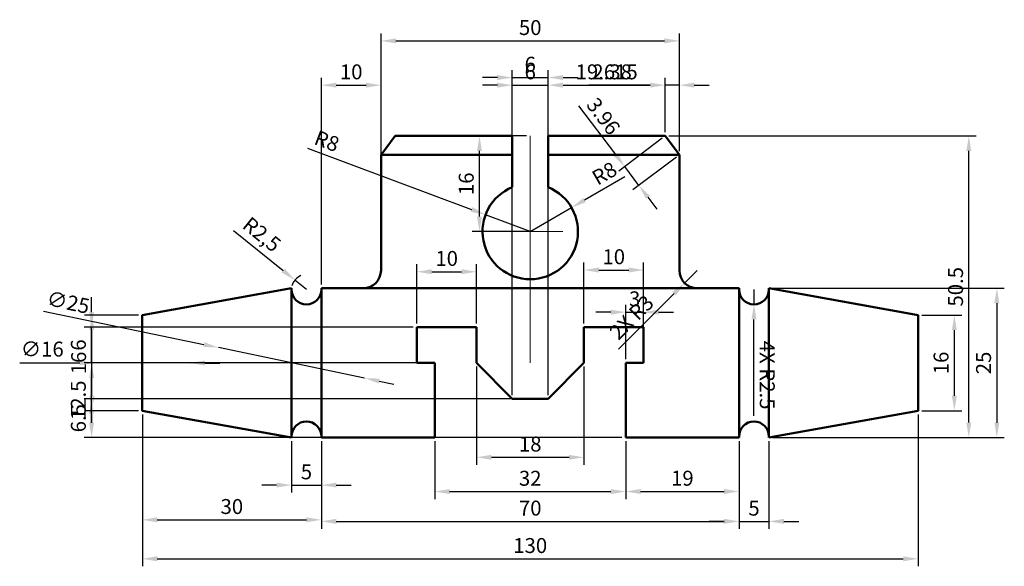
# Model space of a CAD drawing. Units: millimetres. Extents: x 4064 to 4229, y 716 to 807.
import ezdxf

# ---------------------------------------------------------------- set-up
doc = ezdxf.new("R2010")
doc.units = ezdxf.units.MM
doc.linetypes.add('CENTER', pattern=[50.8, 31.75, -6.35, 6.35, -6.35])
for name, color, linetype, lineweight in [('M-CNTR', 4, 'CENTER', 18), ('M-DIMS', 2, 'Continuous', 25), ('M-OUTL', 7, 'Continuous', 50)]:
    doc.layers.add(name, color=color, linetype=linetype, lineweight=lineweight)
doc.styles.get("Standard").update_dxf_attribs({"font": 'arial.ttf'})
doc.dimstyles.new('ISO-25', dxfattribs={"dimtxt": 2.5, "dimasz": 2.5, "dimexe": 1.25, "dimexo": 0.625, "dimtad": 1, "dimtxsty": 'Standard', "dimcen": 2.5, "dimadec": 0, "dimazin": 0, "dimtfac": 1, "dimtmove": 0, "dimatfit": 3, "dimfxl": 1, "dimarcsym": 0})

# ---------------------------------------------------------------- blocks, each defined once
blk = doc.blocks.new('*D1')
at = {"layer": 'Defpoints', "color": 0, "transparency": 16777216}
for p in [(4174.35, 803.87), (4124.35, 784.79), (4174.35, 784.79)]:
    blk.add_point(p, dxfattribs=at)
at = {"layer": 'M-DIMS', "color": 0, "lineweight": -2, "transparency": 16777216}
for p, q in [((4124.35, 785.42), (4124.35, 805.12)), ((4126.85, 803.87), (4171.85, 803.87)), ((4174.35, 785.42), (4174.35, 805.12))]:
    blk.add_line(p, q, dxfattribs=at)
at = {"layer": 'M-DIMS', "color": 0, "transparency": 16777216}
for points in [[(4126.85, 804.29), (4126.85, 803.45), (4124.35, 803.87)], [(4171.85, 804.29), (4171.85, 803.45), (4174.35, 803.87)]]:
    blk.add_solid(points, dxfattribs=at)
at = {"layer": 'M-DIMS', "color": 0, "transparency": 16777216, "insert": (4149.35, 805.77), "char_height": 2.5, "attachment_point": 5}
blk.add_mtext('50', dxfattribs=at)
blk = doc.blocks.new('*D2')
at = {"layer": 'Defpoints', "color": 0, "transparency": 16777216}
for p in [(4152.35, 797.73), (4146.35, 787.95), (4152.35, 787.95)]:
    blk.add_point(p, dxfattribs=at)
at = {"layer": 'M-DIMS', "color": 0, "lineweight": -2, "transparency": 16777216}
for p, q in [((4146.35, 788.58), (4146.35, 798.98)), ((4152.35, 788.58), (4152.35, 798.98)), ((4143.85, 797.73), (4141.35, 797.73)), ((4146.35, 797.73), (4152.35, 797.73)), ((4154.85, 797.73), (4157.35, 797.73))]:
    blk.add_line(p, q, dxfattribs=at)
at = {"layer": 'M-DIMS', "color": 0, "transparency": 16777216}
for points in [[(4143.85, 798.15), (4143.85, 797.32), (4146.35, 797.73)], [(4154.85, 798.15), (4154.85, 797.32), (4152.35, 797.73)]]:
    blk.add_solid(points, dxfattribs=at)
at = {"layer": 'M-DIMS', "color": 0, "transparency": 16777216, "insert": (4149.35, 799.63), "char_height": 2.5, "attachment_point": 5}
blk.add_mtext('6', dxfattribs=at)
blk = doc.blocks.new('*D3')
at = {"layer": 'Defpoints', "color": 0, "transparency": 16777216}
for p in [(4140.35, 749.95), (4158.35, 749.95), (4158.35, 734.15)]:
    blk.add_point(p, dxfattribs=at)
at = {"layer": 'M-DIMS', "color": 0, "lineweight": -2, "transparency": 16777216}
for p, q in [((4140.35, 749.33), (4140.35, 732.9)), ((4158.35, 749.33), (4158.35, 732.9)), ((4142.85, 734.15), (4155.85, 734.15))]:
    blk.add_line(p, q, dxfattribs=at)
at = {"layer": 'M-DIMS', "color": 0, "transparency": 16777216}
for points in [[(4142.85, 734.57), (4142.85, 733.74), (4140.35, 734.15)], [(4155.85, 734.57), (4155.85, 733.74), (4158.35, 734.15)]]:
    blk.add_solid(points, dxfattribs=at)
at = {"layer": 'M-DIMS', "color": 0, "transparency": 16777216, "insert": (4149.35, 736.05), "char_height": 2.5, "attachment_point": 5}
blk.add_mtext('18', dxfattribs=at)
blk = doc.blocks.new('*D4')
at = {"layer": 'Defpoints', "color": 0, "transparency": 16777216}
for p in [(4133.35, 737.45), (4165.35, 737.45), (4165.35, 728.42)]:
    blk.add_point(p, dxfattribs=at)
at = {"layer": 'M-DIMS', "color": 0, "lineweight": -2, "transparency": 16777216}
for p, q in [((4133.35, 736.83), (4133.35, 727.17)), ((4165.35, 736.83), (4165.35, 727.17)), ((4135.85, 728.42), (4162.85, 728.42))]:
    blk.add_line(p, q, dxfattribs=at)
at = {"layer": 'M-DIMS', "color": 0, "transparency": 16777216}
for points in [[(4135.85, 728.84), (4135.85, 728), (4133.35, 728.42)], [(4162.85, 728.84), (4162.85, 728), (4165.35, 728.42)]]:
    blk.add_solid(points, dxfattribs=at)
at = {"layer": 'M-DIMS', "color": 0, "transparency": 16777216, "insert": (4149.35, 730.32), "char_height": 2.5, "attachment_point": 5}
blk.add_mtext('32', dxfattribs=at)
blk = doc.blocks.new('*D5')
at = {"layer": 'Defpoints', "color": 0, "transparency": 16777216}
for p in [(4165.35, 737.45), (4184.35, 737.45), (4184.35, 728.43)]:
    blk.add_point(p, dxfattribs=at)
at = {"layer": 'M-DIMS', "color": 0, "lineweight": -2, "transparency": 16777216}
for p, q in [((4165.35, 736.83), (4165.35, 727.18)), ((4184.35, 736.83), (4184.35, 727.18)), ((4167.85, 728.43), (4181.85, 728.43))]:
    blk.add_line(p, q, dxfattribs=at)
at = {"layer": 'M-DIMS', "color": 0, "transparency": 16777216}
for points in [[(4167.85, 728.85), (4167.85, 728.01), (4165.35, 728.43)], [(4181.85, 728.85), (4181.85, 728.01), (4184.35, 728.43)]]:
    blk.add_solid(points, dxfattribs=at)
at = {"layer": 'M-DIMS', "color": 0, "transparency": 16777216, "insert": (4174.85, 730.33), "char_height": 2.5, "attachment_point": 5}
blk.add_mtext('19', dxfattribs=at)
blk = doc.blocks.new('*D6')
at = {"layer": 'Defpoints', "color": 0, "transparency": 16777216}
for p in [(4114.35, 737.45), (4184.35, 737.45), (4184.35, 723.43)]:
    blk.add_point(p, dxfattribs=at)
at = {"layer": 'M-DIMS', "color": 0, "lineweight": -2, "transparency": 16777216}
for p, q in [((4114.35, 736.83), (4114.35, 722.18)), ((4184.35, 736.83), (4184.35, 722.18)), ((4116.85, 723.43), (4181.85, 723.43))]:
    blk.add_line(p, q, dxfattribs=at)
at = {"layer": 'M-DIMS', "color": 0, "transparency": 16777216}
for points in [[(4116.85, 723.85), (4116.85, 723.01), (4114.35, 723.43)], [(4181.85, 723.85), (4181.85, 723.01), (4184.35, 723.43)]]:
    blk.add_solid(points, dxfattribs=at)
at = {"layer": 'M-DIMS', "color": 0, "transparency": 16777216, "insert": (4149.35, 725.33), "char_height": 2.5, "attachment_point": 5}
blk.add_mtext('70', dxfattribs=at)
blk = doc.blocks.new('*D7')
at = {"layer": 'Defpoints', "color": 0, "transparency": 16777216}
for p in [(4184.35, 737.45), (4189.35, 737.45), (4189.35, 723.42)]:
    blk.add_point(p, dxfattribs=at)
at = {"layer": 'M-DIMS', "color": 0, "lineweight": -2, "transparency": 16777216}
for p, q in [((4184.35, 736.83), (4184.35, 722.17)), ((4189.35, 736.83), (4189.35, 722.17)), ((4181.85, 723.42), (4179.35, 723.42)), ((4184.35, 723.42), (4189.35, 723.42)), ((4191.85, 723.42), (4194.35, 723.42))]:
    blk.add_line(p, q, dxfattribs=at)
at = {"layer": 'M-DIMS', "color": 0, "transparency": 16777216}
for points in [[(4181.85, 723.84), (4181.85, 723.01), (4184.35, 723.42)], [(4191.85, 723.84), (4191.85, 723.01), (4189.35, 723.42)]]:
    blk.add_solid(points, dxfattribs=at)
at = {"layer": 'M-DIMS', "color": 0, "transparency": 16777216, "insert": (4186.85, 725.32), "char_height": 2.5, "attachment_point": 5}
blk.add_mtext('5', dxfattribs=at)
blk = doc.blocks.new('*D8')
at = {"layer": 'Defpoints', "color": 0, "transparency": 16777216}
for p in [(4109.35, 737.46), (4114.35, 737.45), (4114.35, 729.5)]:
    blk.add_point(p, dxfattribs=at)
at = {"layer": 'M-DIMS', "color": 0, "lineweight": -2, "transparency": 16777216}
for p, q in [((4109.35, 736.83), (4109.35, 728.25)), ((4114.35, 736.83), (4114.35, 728.25)), ((4106.85, 729.5), (4104.35, 729.5)), ((4109.35, 729.5), (4114.35, 729.5)), ((4116.85, 729.5), (4119.35, 729.5))]:
    blk.add_line(p, q, dxfattribs=at)
at = {"layer": 'M-DIMS', "color": 0, "transparency": 16777216}
for points in [[(4106.85, 729.92), (4106.85, 729.09), (4109.35, 729.5)], [(4116.85, 729.92), (4116.85, 729.09), (4114.35, 729.5)]]:
    blk.add_solid(points, dxfattribs=at)
at = {"layer": 'M-DIMS', "color": 0, "transparency": 16777216, "insert": (4111.85, 731.4), "char_height": 2.5, "attachment_point": 5}
blk.add_mtext('5', dxfattribs=at)
blk = doc.blocks.new('*D9')
at = {"layer": 'Defpoints', "color": 0, "transparency": 16777216}
for p in [(4084.35, 741.95), (4114.35, 737.45), (4114.35, 723.69)]:
    blk.add_point(p, dxfattribs=at)
at = {"layer": 'M-DIMS', "color": 0, "lineweight": -2, "transparency": 16777216}
for p, q in [((4084.35, 741.33), (4084.35, 722.44)), ((4114.35, 736.83), (4114.35, 722.44)), ((4086.85, 723.69), (4111.85, 723.69))]:
    blk.add_line(p, q, dxfattribs=at)
at = {"layer": 'M-DIMS', "color": 0, "transparency": 16777216}
for points in [[(4086.85, 724.1), (4086.85, 723.27), (4084.35, 723.69)], [(4111.85, 724.1), (4111.85, 723.27), (4114.35, 723.69)]]:
    blk.add_solid(points, dxfattribs=at)
at = {"layer": 'M-DIMS', "color": 0, "transparency": 16777216, "insert": (4099.35, 725.59), "char_height": 2.5, "attachment_point": 5}
blk.add_mtext('30', dxfattribs=at)
blk = doc.blocks.new('*D10')
at = {"layer": 'Defpoints', "color": 0, "transparency": 16777216}
for p in [(4084.35, 741.95), (4214.35, 741.95), (4214.35, 717.16)]:
    blk.add_point(p, dxfattribs=at)
at = {"layer": 'M-DIMS', "color": 0, "lineweight": -2, "transparency": 16777216}
for p, q in [((4084.35, 741.33), (4084.35, 715.91)), ((4214.35, 741.33), (4214.35, 715.91)), ((4086.85, 717.16), (4211.85, 717.16))]:
    blk.add_line(p, q, dxfattribs=at)
at = {"layer": 'M-DIMS', "color": 0, "transparency": 16777216}
for points in [[(4086.85, 717.58), (4086.85, 716.74), (4084.35, 717.16)], [(4211.85, 717.58), (4211.85, 716.74), (4214.35, 717.16)]]:
    blk.add_solid(points, dxfattribs=at)
at = {"layer": 'M-DIMS', "color": 0, "transparency": 16777216, "insert": (4149.35, 719.06), "char_height": 2.5, "attachment_point": 5}
blk.add_mtext('130', dxfattribs=at)
blk = doc.blocks.new('*D11')
at = {"layer": 'Defpoints', "color": 0, "transparency": 16777216}
for p in [(4076.35, 749.97), (4092.35, 749.94)]:
    blk.add_point(p, dxfattribs=at)
at = {"layer": 'M-DIMS', "color": 0, "lineweight": -2, "transparency": 16777216}
for p, q in [((4063.8, 749.99), (4073.85, 749.97)), ((4092.35, 749.94), (4076.35, 749.97)), ((4094.85, 749.94), (4097.35, 749.93))]:
    blk.add_line(p, q, dxfattribs=at)
at = {"layer": 'M-DIMS', "color": 0, "transparency": 16777216}
for points in [[(4073.85, 750.39), (4073.85, 749.55), (4076.35, 749.97)], [(4094.85, 750.35), (4094.85, 749.52), (4092.35, 749.94)]]:
    blk.add_solid(points, dxfattribs=at)
at = {"layer": 'M-DIMS', "color": 0, "transparency": 16777216, "insert": (4067.58, 751.95), "char_height": 2.5, "attachment_point": 5, "rotation": 359.9089}
blk.add_mtext('∅16', dxfattribs=at)
blk = doc.blocks.new('*D12')
at = {"layer": 'Defpoints', "color": 0, "transparency": 16777216}
for p in [(4097.11, 752.52), (4121.58, 747.42)]:
    blk.add_point(p, dxfattribs=at)
at = {"layer": 'M-DIMS', "color": 0, "lineweight": -2, "transparency": 16777216}
for p, q in [((4067.77, 758.64), (4094.66, 753.03)), ((4121.58, 747.42), (4097.11, 752.52)), ((4124.03, 746.91), (4126.48, 746.4))]:
    blk.add_line(p, q, dxfattribs=at)
at = {"layer": 'M-DIMS', "color": 0, "transparency": 16777216}
for points in [[(4094.75, 753.44), (4094.58, 752.63), (4097.11, 752.52)], [(4124.12, 747.32), (4123.95, 746.51), (4121.58, 747.42)]]:
    blk.add_solid(points, dxfattribs=at)
at = {"layer": 'M-DIMS', "color": 0, "transparency": 16777216, "insert": (4071.87, 759.79), "char_height": 2.5, "attachment_point": 5, "rotation": 348.232}
blk.add_mtext('∅25', dxfattribs=at)
blk = doc.blocks.new('*D13')
at = {"layer": 'Defpoints', "color": 0, "transparency": 16777216}
for p in [(4075.9, 757.95), (4084.35, 757.95), (4084.35, 741.95)]:
    blk.add_point(p, dxfattribs=at)
at = {"layer": 'M-DIMS', "color": 0, "lineweight": -2, "transparency": 16777216}
for p, q in [((4083.72, 757.95), (4074.65, 757.95)), ((4075.9, 744.45), (4075.9, 755.45)), ((4083.72, 741.95), (4074.65, 741.95))]:
    blk.add_line(p, q, dxfattribs=at)
at = {"layer": 'M-DIMS', "color": 0, "transparency": 16777216}
for points in [[(4075.49, 755.45), (4076.32, 755.45), (4075.9, 757.95)], [(4075.49, 744.45), (4076.32, 744.45), (4075.9, 741.95)]]:
    blk.add_solid(points, dxfattribs=at)
at = {"layer": 'M-DIMS', "color": 0, "transparency": 16777216, "insert": (4074, 749.95), "char_height": 2.5, "attachment_point": 5, "rotation": 90}
blk.add_mtext('16', dxfattribs=at)
blk = doc.blocks.new('*D14')
at = {"layer": 'Defpoints', "color": 0, "transparency": 16777216}
for p in [(4168.35, 765.51), (4158.35, 755.95), (4168.35, 755.95)]:
    blk.add_point(p, dxfattribs=at)
at = {"layer": 'M-DIMS', "color": 0, "lineweight": -2, "transparency": 16777216}
for p, q in [((4158.35, 756.58), (4158.35, 766.76)), ((4168.35, 756.58), (4168.35, 766.76)), ((4160.85, 765.51), (4165.85, 765.51))]:
    blk.add_line(p, q, dxfattribs=at)
at = {"layer": 'M-DIMS', "color": 0, "transparency": 16777216}
for points in [[(4160.85, 765.93), (4160.85, 765.09), (4158.35, 765.51)], [(4165.85, 765.93), (4165.85, 765.09), (4168.35, 765.51)]]:
    blk.add_solid(points, dxfattribs=at)
at = {"layer": 'M-DIMS', "color": 0, "transparency": 16777216, "insert": (4163.35, 767.41), "char_height": 2.5, "attachment_point": 5}
blk.add_mtext('10', dxfattribs=at)
blk = doc.blocks.new('*D15')
at = {"layer": 'Defpoints', "color": 0, "transparency": 16777216}
for p in [(4140.35, 765.22), (4130.35, 755.95), (4140.35, 755.95)]:
    blk.add_point(p, dxfattribs=at)
at = {"layer": 'M-DIMS', "color": 0, "lineweight": -2, "transparency": 16777216}
for p, q in [((4130.35, 756.58), (4130.35, 766.47)), ((4140.35, 756.58), (4140.35, 766.47)), ((4132.85, 765.22), (4137.85, 765.22))]:
    blk.add_line(p, q, dxfattribs=at)
at = {"layer": 'M-DIMS', "color": 0, "transparency": 16777216}
for points in [[(4132.85, 765.64), (4132.85, 764.8), (4130.35, 765.22)], [(4137.85, 765.64), (4137.85, 764.8), (4140.35, 765.22)]]:
    blk.add_solid(points, dxfattribs=at)
at = {"layer": 'M-DIMS', "color": 0, "transparency": 16777216, "insert": (4135.35, 767.12), "char_height": 2.5, "attachment_point": 5}
blk.add_mtext('10', dxfattribs=at)
blk = doc.blocks.new('*D16')
at = {"layer": 'Defpoints', "color": 0, "transparency": 16777216}
for p in [(4141.86, 774.76), (4149.35, 771.95)]:
    blk.add_point(p, dxfattribs=at)
at = {"layer": 'M-DIMS', "color": 0, "lineweight": -2, "transparency": 16777216}
for p, q in [((4112.02, 785.93), (4139.51, 775.64)), ((4149.35, 771.95), (4141.86, 774.76))]:
    blk.add_line(p, q, dxfattribs=at)
at = {"layer": 'M-DIMS', "color": 0, "transparency": 16777216}
blk.add_solid([(4139.66, 776.03), (4139.37, 775.25), (4141.86, 774.76)], dxfattribs=at)
at = {"layer": 'M-DIMS', "color": 0, "transparency": 16777216, "insert": (4115.17, 786.79), "char_height": 2.5, "attachment_point": 5, "rotation": 339.4696}
blk.add_mtext('R8', dxfattribs=at)
blk = doc.blocks.new('*D17')
at = {"layer": 'Defpoints', "color": 0, "transparency": 16777216}
for p in [(4214.35, 757.95), (4214.35, 741.95), (4220.42, 741.95)]:
    blk.add_point(p, dxfattribs=at)
at = {"layer": 'M-DIMS', "color": 0, "lineweight": -2, "transparency": 16777216}
for p, q in [((4214.97, 757.95), (4221.67, 757.95)), ((4220.42, 755.45), (4220.42, 744.45)), ((4214.97, 741.95), (4221.67, 741.95))]:
    blk.add_line(p, q, dxfattribs=at)
at = {"layer": 'M-DIMS', "color": 0, "transparency": 16777216}
for points in [[(4220.01, 755.45), (4220.84, 755.45), (4220.42, 757.95)], [(4220.01, 744.45), (4220.84, 744.45), (4220.42, 741.95)]]:
    blk.add_solid(points, dxfattribs=at)
at = {"layer": 'M-DIMS', "color": 0, "transparency": 16777216, "insert": (4218.52, 749.95), "char_height": 2.5, "attachment_point": 5, "rotation": 90}
blk.add_mtext('16', dxfattribs=at)
blk = doc.blocks.new('*D18')
at = {"layer": 'Defpoints', "color": 0, "transparency": 16777216}
for p in [(4189.35, 762.45), (4189.35, 737.45), (4227.55, 737.45)]:
    blk.add_point(p, dxfattribs=at)
at = {"layer": 'M-DIMS', "color": 0, "lineweight": -2, "transparency": 16777216}
for p, q in [((4189.97, 762.45), (4228.8, 762.45)), ((4227.55, 759.95), (4227.55, 739.95)), ((4189.97, 737.45), (4228.8, 737.45))]:
    blk.add_line(p, q, dxfattribs=at)
at = {"layer": 'M-DIMS', "color": 0, "transparency": 16777216}
for points in [[(4227.13, 759.95), (4227.96, 759.95), (4227.55, 762.45)], [(4227.13, 739.95), (4227.96, 739.95), (4227.55, 737.45)]]:
    blk.add_solid(points, dxfattribs=at)
at = {"layer": 'M-DIMS', "color": 0, "transparency": 16777216, "insert": (4225.64, 749.95), "char_height": 2.5, "attachment_point": 5, "rotation": 90}
blk.add_mtext('25', dxfattribs=at)
blk = doc.blocks.new('*D19')
at = {"layer": 'Defpoints', "color": 0, "transparency": 16777216}
for p in [(4109.91, 763.83), (4111.85, 762.25)]:
    blk.add_point(p, dxfattribs=at)
at = {"layer": 'M-DIMS', "color": 0, "lineweight": -2, "transparency": 16777216}
for p, q in [((4099.65, 772.15), (4107.96, 765.4)), ((4111.85, 762.25), (4109.91, 763.83))]:
    blk.add_line(p, q, dxfattribs=at)
blk.add_arc((4111.85, 762.25), 2.5, 112.2968, 165.6761, dxfattribs=at)
at = {"layer": 'M-DIMS', "color": 0, "transparency": 16777216}
blk.add_solid([(4108.23, 765.73), (4107.7, 765.08), (4109.91, 763.83)], dxfattribs=at)
at = {"layer": 'M-DIMS', "color": 0, "transparency": 16777216, "insert": (4104.18, 771.22), "char_height": 2.5, "attachment_point": 5, "rotation": 320.9447}
blk.add_mtext('R2,5', dxfattribs=at)
blk = doc.blocks.new('STUD-END-TAPERED')
for p, q in [((5, 12.5), (5, -12.5)), ((5, 12.5), (30, 8)), ((30, -8), (30, 8)), ((30, 0), (30, 8)), ((30, 8), (30, -8)), ((5, -12.5), (30, -8))]:
    blk.add_line(p, q)
for centre, start, end in [((2.5, 12.3), 180, 0), ((2.5, -12.3), 0, 180)]:
    blk.add_arc(centre, 2.5, start, end)
blk = doc.blocks.new('*D21')
at = {"layer": 'Defpoints', "color": 0, "transparency": 16777216}
for p in [(4171.96, 787.95), (4222.85, 787.95), (4189.35, 737.46)]:
    blk.add_point(p, dxfattribs=at)
at = {"layer": 'M-DIMS', "color": 0, "lineweight": -2, "transparency": 16777216}
for p, q in [((4172.59, 787.95), (4224.1, 787.95)), ((4222.85, 739.96), (4222.85, 785.45)), ((4189.97, 737.46), (4224.1, 737.46))]:
    blk.add_line(p, q, dxfattribs=at)
at = {"layer": 'M-DIMS', "color": 0, "transparency": 16777216}
for points in [[(4222.43, 785.45), (4223.26, 785.45), (4222.85, 787.95)], [(4222.43, 739.96), (4223.26, 739.96), (4222.85, 737.46)]]:
    blk.add_solid(points, dxfattribs=at)
at = {"layer": 'M-DIMS', "color": 0, "transparency": 16777216, "insert": (4220.95, 762.7), "char_height": 2.5, "attachment_point": 5, "rotation": 90}
blk.add_mtext('50.5', dxfattribs=at)
blk = doc.blocks.new('*D22')
at = {"layer": 'Defpoints', "color": 0, "transparency": 16777216}
for p in [(4140.85, 787.95), (4149.35, 787.95), (4149.35, 771.95)]:
    blk.add_point(p, dxfattribs=at)
at = {"layer": 'M-DIMS', "color": 0, "lineweight": -2, "transparency": 16777216}
for p, q in [((4148.72, 787.95), (4139.6, 787.95)), ((4140.85, 774.45), (4140.85, 785.45)), ((4148.72, 771.95), (4139.6, 771.95))]:
    blk.add_line(p, q, dxfattribs=at)
at = {"layer": 'M-DIMS', "color": 0, "transparency": 16777216}
for points in [[(4140.43, 785.45), (4141.26, 785.45), (4140.85, 787.95)], [(4140.43, 774.45), (4141.26, 774.45), (4140.85, 771.95)]]:
    blk.add_solid(points, dxfattribs=at)
at = {"layer": 'M-DIMS', "color": 0, "transparency": 16777216, "insert": (4138.95, 779.95), "char_height": 2.5, "attachment_point": 5, "rotation": 90}
blk.add_mtext('16', dxfattribs=at)
blk = doc.blocks.new('*D23')
at = {"layer": 'Defpoints', "color": 0, "transparency": 16777216}
for p in [(4171.96, 787.95), (4174.35, 784.79), (4165.18, 782.83)]:
    blk.add_point(p, dxfattribs=at)
at = {"layer": 'M-DIMS', "color": 0, "lineweight": -2, "transparency": 16777216}
for p, q in [((4163.67, 784.83), (4157.5, 793)), ((4171.46, 787.58), (4164.18, 782.08)), ((4173.85, 784.42), (4166.57, 778.92)), ((4167.56, 779.67), (4165.18, 782.83)), ((4169.07, 777.68), (4170.58, 775.68))]:
    blk.add_line(p, q, dxfattribs=at)
at = {"layer": 'M-DIMS', "color": 0, "transparency": 16777216}
for points in [[(4164, 785.08), (4163.34, 784.58), (4165.18, 782.83)], [(4169.4, 777.93), (4168.74, 777.43), (4167.56, 779.67)]]:
    blk.add_solid(points, dxfattribs=at)
at = {"layer": 'M-DIMS', "color": 0, "transparency": 16777216, "insert": (4161.35, 791.06), "char_height": 2.5, "attachment_point": 5, "rotation": 307.0443}
blk.add_mtext('3.96', dxfattribs=at)
blk = doc.blocks.new('*D24')
at = {"layer": 'Defpoints', "color": 0, "transparency": 16777216}
for p in [(4171.96, 796.45), (4171.96, 787.95), (4174.35, 784.79)]:
    blk.add_point(p, dxfattribs=at)
at = {"layer": 'M-DIMS', "color": 0, "lineweight": -2, "transparency": 16777216}
for p, q in [((4171.96, 788.58), (4171.96, 797.7)), ((4174.35, 785.42), (4174.35, 797.7)), ((4169.46, 796.45), (4159.17, 796.45)), ((4174.35, 796.45), (4171.96, 796.45)), ((4176.85, 796.45), (4179.35, 796.45))]:
    blk.add_line(p, q, dxfattribs=at)
at = {"layer": 'M-DIMS', "color": 0, "transparency": 16777216}
for points in [[(4169.46, 796.87), (4169.46, 796.04), (4171.96, 796.45)], [(4176.85, 796.87), (4176.85, 796.04), (4174.35, 796.45)]]:
    blk.add_solid(points, dxfattribs=at)
at = {"layer": 'M-DIMS', "color": 0, "transparency": 16777216, "insert": (4163.07, 798.36), "char_height": 2.5, "attachment_point": 5}
blk.add_mtext('2.38', dxfattribs=at)
blk = doc.blocks.new('*D25')
at = {"layer": 'Defpoints', "color": 0, "transparency": 16777216}
for p in [(4075.85, 749.95), (4133.35, 749.95), (4133.35, 737.45)]:
    blk.add_point(p, dxfattribs=at)
at = {"layer": 'M-DIMS', "color": 0, "lineweight": -2, "transparency": 16777216}
for p, q in [((4132.72, 749.95), (4074.6, 749.95)), ((4075.85, 739.95), (4075.85, 747.45)), ((4132.72, 737.45), (4074.6, 737.45))]:
    blk.add_line(p, q, dxfattribs=at)
at = {"layer": 'M-DIMS', "color": 0, "transparency": 16777216}
for points in [[(4075.43, 747.45), (4076.26, 747.45), (4075.85, 749.95)], [(4075.43, 739.95), (4076.26, 739.95), (4075.85, 737.45)]]:
    blk.add_solid(points, dxfattribs=at)
at = {"layer": 'M-DIMS', "color": 0, "transparency": 16777216, "insert": (4073.95, 743.7), "char_height": 2.5, "attachment_point": 5, "rotation": 90}
blk.add_mtext('12.5', dxfattribs=at)
blk = doc.blocks.new('*D26')
at = {"layer": 'Defpoints', "color": 0, "transparency": 16777216}
for p in [(4075.85, 755.95), (4130.35, 755.95), (4130.35, 749.95)]:
    blk.add_point(p, dxfattribs=at)
at = {"layer": 'M-DIMS', "color": 0, "lineweight": -2, "transparency": 16777216}
for p, q in [((4075.85, 758.45), (4075.85, 760.95)), ((4129.72, 755.95), (4074.6, 755.95)), ((4075.85, 749.95), (4075.85, 755.95)), ((4129.72, 749.95), (4074.6, 749.95)), ((4075.85, 747.45), (4075.85, 744.95))]:
    blk.add_line(p, q, dxfattribs=at)
at = {"layer": 'M-DIMS', "color": 0, "transparency": 16777216}
for points in [[(4075.43, 758.45), (4076.26, 758.45), (4075.85, 755.95)], [(4075.43, 747.45), (4076.26, 747.45), (4075.85, 749.95)]]:
    blk.add_solid(points, dxfattribs=at)
at = {"layer": 'M-DIMS', "color": 0, "transparency": 16777216, "insert": (4073.95, 752.95), "char_height": 2.5, "attachment_point": 5, "rotation": 90}
blk.add_mtext('6', dxfattribs=at)
blk = doc.blocks.new('*D27')
at = {"layer": 'Defpoints', "color": 0, "transparency": 16777216}
for p in [(4152.35, 743.95), (4075.85, 737.45), (4165.35, 737.45)]:
    blk.add_point(p, dxfattribs=at)
at = {"layer": 'M-DIMS', "color": 0, "lineweight": -2, "transparency": 16777216}
for p, q in [((4151.72, 743.95), (4074.6, 743.95)), ((4075.85, 741.45), (4075.85, 739.95)), ((4164.72, 737.45), (4074.6, 737.45))]:
    blk.add_line(p, q, dxfattribs=at)
at = {"layer": 'M-DIMS', "color": 0, "transparency": 16777216}
for points in [[(4075.43, 741.45), (4076.26, 741.45), (4075.85, 743.95)], [(4075.43, 739.95), (4076.26, 739.95), (4075.85, 737.45)]]:
    blk.add_solid(points, dxfattribs=at)
at = {"layer": 'M-DIMS', "color": 0, "transparency": 16777216, "insert": (4073.95, 740.7), "char_height": 2.5, "attachment_point": 5, "rotation": 90}
blk.add_mtext('6.5', dxfattribs=at)
blk = doc.blocks.new('*D28')
at = {"layer": 'Defpoints', "color": 0, "transparency": 16777216}
for p in [(4152.35, 796.45), (4146.35, 743.95), (4152.35, 743.95)]:
    blk.add_point(p, dxfattribs=at)
at = {"layer": 'M-DIMS', "color": 0, "lineweight": -2, "transparency": 16777216}
for p, q in [((4146.35, 744.58), (4146.35, 797.7)), ((4152.35, 744.58), (4152.35, 797.7)), ((4143.85, 796.45), (4141.35, 796.45)), ((4146.35, 796.45), (4152.35, 796.45)), ((4154.85, 796.45), (4157.35, 796.45))]:
    blk.add_line(p, q, dxfattribs=at)
at = {"layer": 'M-DIMS', "color": 0, "transparency": 16777216}
for points in [[(4143.85, 796.87), (4143.85, 796.04), (4146.35, 796.45)], [(4154.85, 796.87), (4154.85, 796.04), (4152.35, 796.45)]]:
    blk.add_solid(points, dxfattribs=at)
at = {"layer": 'M-DIMS', "color": 0, "transparency": 16777216, "insert": (4149.35, 798.36), "char_height": 2.5, "attachment_point": 5}
blk.add_mtext('6', dxfattribs=at)
blk = doc.blocks.new('*D29')
at = {"layer": 'Defpoints', "color": 0, "transparency": 16777216}
for p in [(4124.35, 796.45), (4124.35, 765.45), (4114.35, 762.45)]:
    blk.add_point(p, dxfattribs=at)
at = {"layer": 'M-DIMS', "color": 0, "lineweight": -2, "transparency": 16777216}
for p, q in [((4114.35, 763.08), (4114.35, 797.7)), ((4124.35, 766.08), (4124.35, 797.7)), ((4116.85, 796.45), (4121.85, 796.45))]:
    blk.add_line(p, q, dxfattribs=at)
at = {"layer": 'M-DIMS', "color": 0, "transparency": 16777216}
for points in [[(4116.85, 796.87), (4116.85, 796.04), (4114.35, 796.45)], [(4121.85, 796.87), (4121.85, 796.04), (4124.35, 796.45)]]:
    blk.add_solid(points, dxfattribs=at)
at = {"layer": 'M-DIMS', "color": 0, "transparency": 16777216, "insert": (4119.35, 798.36), "char_height": 2.5, "attachment_point": 5}
blk.add_mtext('10', dxfattribs=at)
blk = doc.blocks.new('*D30')
at = {"layer": 'Defpoints', "color": 0, "transparency": 16777216}
for p in [(4171.96, 796.45), (4152.35, 787.95), (4171.96, 787.95)]:
    blk.add_point(p, dxfattribs=at)
at = {"layer": 'M-DIMS', "color": 0, "lineweight": -2, "transparency": 16777216}
for p, q in [((4152.35, 788.58), (4152.35, 797.7)), ((4171.96, 788.58), (4171.96, 797.7)), ((4154.85, 796.45), (4169.46, 796.45))]:
    blk.add_line(p, q, dxfattribs=at)
at = {"layer": 'M-DIMS', "color": 0, "transparency": 16777216}
for points in [[(4154.85, 796.87), (4154.85, 796.04), (4152.35, 796.45)], [(4169.46, 796.87), (4169.46, 796.04), (4171.96, 796.45)]]:
    blk.add_solid(points, dxfattribs=at)
at = {"layer": 'M-DIMS', "color": 0, "transparency": 16777216, "insert": (4162.16, 798.36), "char_height": 2.5, "attachment_point": 5}
blk.add_mtext('19.615', dxfattribs=at)
blk = doc.blocks.new('*D31')
at = {"layer": 'Defpoints', "color": 0, "transparency": 16777216}
for p in [(4168.35, 758.45), (4165.35, 749.95), (4168.35, 749.95)]:
    blk.add_point(p, dxfattribs=at)
at = {"layer": 'M-DIMS', "color": 0, "lineweight": -2, "transparency": 16777216}
for p, q in [((4165.35, 750.58), (4165.35, 759.7)), ((4168.35, 750.58), (4168.35, 759.7)), ((4162.85, 758.45), (4160.35, 758.45)), ((4165.35, 758.45), (4168.35, 758.45)), ((4170.85, 758.45), (4173.35, 758.45))]:
    blk.add_line(p, q, dxfattribs=at)
at = {"layer": 'M-DIMS', "color": 0, "transparency": 16777216}
for points in [[(4162.85, 758.87), (4162.85, 758.04), (4165.35, 758.45)], [(4170.85, 758.87), (4170.85, 758.04), (4168.35, 758.45)]]:
    blk.add_solid(points, dxfattribs=at)
at = {"layer": 'M-DIMS', "color": 0, "transparency": 16777216, "insert": (4166.85, 760.36), "char_height": 2.5, "attachment_point": 5}
blk.add_mtext('3', dxfattribs=at)
blk = doc.blocks.new('*D32')
at = {"layer": 'Defpoints', "color": 0, "transparency": 16777216}
for p in [(4156.28, 775.95), (4149.35, 771.95)]:
    blk.add_point(p, dxfattribs=at)
at = {"layer": 'M-DIMS', "color": 0, "lineweight": -2, "transparency": 16777216}
for p, q in [((4165.19, 781.09), (4158.44, 777.2)), ((4149.35, 771.95), (4156.28, 775.95))]:
    blk.add_line(p, q, dxfattribs=at)
at = {"layer": 'M-DIMS', "color": 0, "transparency": 16777216}
blk.add_solid([(4158.24, 777.56), (4158.65, 776.84), (4156.28, 775.95)], dxfattribs=at)
at = {"layer": 'M-DIMS', "color": 0, "transparency": 16777216, "insert": (4161.95, 781.41), "char_height": 2.5, "attachment_point": 5, "rotation": 29.9603}
blk.add_mtext('R8', dxfattribs=at)
blk = doc.blocks.new('*D33')
at = {"layer": 'Defpoints', "color": 0, "transparency": 16777216}
for p in [(4177.35, 765.45), (4175.23, 763.33)]:
    blk.add_point(p, dxfattribs=at)
at = {"layer": 'M-DIMS', "color": 0, "lineweight": -2, "transparency": 16777216}
for p, q in [((4177.35, 765.45), (4175.23, 763.33)), ((4164.13, 752.24), (4173.46, 761.57))]:
    blk.add_line(p, q, dxfattribs=at)
at = {"layer": 'M-DIMS', "color": 0, "transparency": 16777216}
blk.add_solid([(4173.16, 761.86), (4173.75, 761.27), (4175.23, 763.33)], dxfattribs=at)
at = {"layer": 'M-DIMS', "color": 0, "transparency": 16777216, "insert": (4166.56, 757.36), "char_height": 2.5, "attachment_point": 5, "rotation": 44.9916}
blk.add_mtext('2X R3', dxfattribs=at)
blk = doc.blocks.new('*D34')
at = {"layer": 'Defpoints', "color": 0, "transparency": 16777216}
for p in [(4186.85, 762.25), (4186.85, 759.75)]:
    blk.add_point(p, dxfattribs=at)
at = {"layer": 'M-DIMS', "color": 0, "lineweight": -2, "transparency": 16777216}
for p, q in [((4186.85, 762.25), (4186.85, 759.75)), ((4186.85, 741.07), (4186.85, 757.25))]:
    blk.add_line(p, q, dxfattribs=at)
at = {"layer": 'M-DIMS', "color": 0, "transparency": 16777216}
blk.add_solid([(4187.27, 757.25), (4186.43, 757.25), (4186.85, 759.75)], dxfattribs=at)
at = {"layer": 'M-DIMS', "color": 0, "transparency": 16777216, "insert": (4188.75, 747.91), "char_height": 2.5, "attachment_point": 5, "rotation": 270.0094}
blk.add_mtext('4X R2.5', dxfattribs=at)

msp = doc.modelspace()

# ---------------------------------------------------------------- linework, layer by layer
at = {"layer": 'M-CNTR'}
for p, q in [((4149.3476, 749.954), (4149.3476, 787.954)), ((4149.3476, 787.954), (4149.3476, 771.954)), ((4154.7996, 771.954), (4144.1085, 771.954)), ((4149.3476, 771.954), (4154.7996, 771.954))]:
    msp.add_line(p, q, dxfattribs=at)
at = {"layer": 'M-OUTL'}
for p, q in [((4124.3476, 784.7944), (4126.7323, 787.954)), ((4146.3476, 787.954), (4126.7323, 787.954)), ((4146.3476, 787.954), (4146.3476, 779.3702)), ((4152.3476, 787.954), (4152.3476, 779.3702)), ((4152.3476, 787.954), (4171.9629, 787.954)), ((4171.9629, 787.954), (4152.3476, 787.954)), ((4174.3476, 784.7944), (4171.9629, 787.954)), ((4124.3476, 784.7944), (4124.3476, 765.454)), ((4146.3476, 784.7944), (4124.3476, 784.7944)), ((4152.3476, 784.7944), (4174.3476, 784.7944)), ((4174.3476, 784.7944), (4152.3476, 784.7944)), ((4174.3476, 784.7944), (4174.3476, 765.454)), ((4114.3476, 737.454), (4114.3476, 762.454)), ((4114.3476, 762.454), (4121.3476, 762.454)), ((4114.3476, 762.454), (4184.3476, 762.454)), ((4177.3476, 762.454), (4184.3476, 762.454)), ((4184.3476, 737.454), (4184.3476, 762.454)), ((4140.3476, 755.954), (4130.3476, 755.954)), ((4130.3476, 755.954), (4130.3476, 749.954)), ((4140.3476, 755.954), (4131.9446, 755.954)), ((4140.3476, 749.954), (4140.3476, 755.954)), ((4158.3476, 755.954), (4168.3476, 755.954)), ((4168.3476, 755.954), (4158.3476, 755.954)), ((4158.3476, 755.954), (4168.3476, 755.954)), ((4158.3476, 755.954), (4168.3476, 755.954)), ((4158.3476, 749.954), (4158.3476, 755.954)), ((4168.3476, 755.954), (4168.3476, 749.954)), ((4130.3476, 749.954), (4133.3476, 749.954)), ((4130.3476, 749.954), (4133.3476, 749.954)), ((4130.3476, 749.954), (4133.3476, 749.954)), ((4133.3476, 737.454), (4133.3476, 749.954)), ((4146.3476, 743.954), (4140.3476, 749.954)), ((4152.3476, 743.954), (4158.3476, 749.954)), ((4165.3476, 743.954), (4165.3476, 749.954)), ((4168.3476, 749.954), (4165.3476, 749.954)), ((4165.3476, 749.954), (4168.3476, 749.954)), ((4165.3476, 749.954), (4168.3476, 749.954)), ((4152.3476, 743.954), (4146.3476, 743.954)), ((4152.3476, 743.954), (4146.3476, 743.954)), ((4149.3476, 743.954), (4152.3476, 743.954)), ((4149.3476, 743.954), (4152.3476, 743.954)), ((4165.3476, 743.954), (4165.3476, 737.454)), ((4133.3476, 737.454), (4114.3476, 737.454)), ((4114.3476, 737.454), (4133.3476, 737.454)), ((4165.3476, 737.454), (4184.3476, 737.454)), ((4165.3476, 737.454), (4184.3476, 737.454))]:
    msp.add_line(p, q, dxfattribs=at)
for centre, radius, start, end in [((4149.3476, 771.954), 8, 112.024313, 67.975687), ((4121.3476, 765.454), 3, 270, 0), ((4177.3476, 765.454), 3, 180, 270)]:
    msp.add_arc(centre, radius, start, end, dxfattribs=at)

# ---------------------------------------------------------------- block references
at = {"layer": 'M-OUTL', "extrusion": (0, 0, -1), "zscale": -1}
msp.add_blockref('STUD-END-TAPERED', (-4114.3476, 749.954), dxfattribs=at)
at = {"layer": 'M-OUTL'}
msp.add_blockref('STUD-END-TAPERED', (4184.3476, 749.954), dxfattribs=at)

# ---------------------------------------------------------------- dimensions: what is measured, and where the dimension line sits
at = {"layer": 'M-DIMS'}
for base, p1, p2, override, picture, middle in [((4174.3476, 803.8701), (4124.3476, 784.7944), (4174.3476, 784.7944), {"dimclrd": 0, "dimclre": 0, "dimclrt": 0}, '*D1', (4149.3476, 805.7716)), ((4152.3476, 797.7334), (4146.3476, 787.954), (4152.3476, 787.954), {"dimclrd": 0, "dimclre": 0, "dimclrt": 0}, '*D2', (4149.3476, 799.6349)), ((4124.3476, 796.454), (4114.3476, 762.454), (4124.3476, 765.454), {"dimdec": 0, "dimlfac": 1, "dimrnd": 0, "dimzin": 0, "dimdsep": 46, "dimlunit": 2}, '*D29', (4119.3476, 798.3554)), ((4152.3476, 796.454), (4146.3476, 743.954), (4152.3476, 743.954), {"dimdec": 0, "dimlfac": 1, "dimrnd": 0, "dimzin": 0, "dimdsep": 46, "dimlunit": 2}, '*D28', (4149.3476, 798.3554)), ((4171.9629, 796.454), (4152.3476, 787.954), (4171.9629, 787.954), {"dimdec": 3, "dimlfac": 1, "dimrnd": 0, "dimzin": 0, "dimdsep": 46, "dimlunit": 2}, '*D30', (4162.1552, 798.3554)), ((4171.9629, 796.454), (4174.3476, 784.7944), (4171.9629, 787.954), {"dimdec": 2, "dimlfac": 1, "dimrnd": 0, "dimzin": 0, "dimdsep": 46, "dimlunit": 2}, '*D24', (4163.0671, 798.3563)), ((4168.3476, 765.5114), (4158.3476, 755.954), (4168.3476, 755.954), {"dimclrd": 0, "dimclre": 0, "dimclrt": 0}, '*D14', (4163.3476, 767.4128)), ((4140.3476, 765.2184), (4130.3476, 755.954), (4140.3476, 755.954), {"dimclrd": 0, "dimclre": 0, "dimclrt": 0}, '*D15', (4135.3476, 767.1198)), ((4158.3476, 734.1529), (4140.3476, 749.954), (4158.3476, 749.954), {"dimclrd": 0, "dimclre": 0, "dimclrt": 0}, '*D3', (4149.3476, 736.0543)), ((4114.3476, 723.6876), (4084.3476, 741.954), (4114.3476, 737.454), {"dimclrd": 0, "dimclre": 0, "dimclrt": 0}, '*D9', (4099.3476, 725.5899)), ((4214.3476, 717.159), (4084.3476, 741.954), (4214.3476, 741.954), {"dimclrd": 0, "dimclre": 0, "dimclrt": 0}, '*D10', (4149.3476, 719.0613)), ((4114.3476, 729.5037), (4109.3476, 737.4554), (4114.3476, 737.454), {"dimclrd": 0, "dimclre": 0, "dimclrt": 0}, '*D8', (4111.8476, 731.4)), ((4184.3476, 723.4285), (4114.3476, 737.454), (4184.3476, 737.454), {"dimclrd": 0, "dimclre": 0, "dimclrt": 0}, '*D6', (4149.3476, 725.3299)), ((4165.3476, 728.4187), (4133.3476, 737.454), (4165.3476, 737.454), {"dimclrd": 0, "dimclre": 0, "dimclrt": 0}, '*D4', (4149.3476, 730.321)), ((4184.3476, 728.4301), (4165.3476, 737.454), (4184.3476, 737.454), {"dimclrd": 0, "dimclre": 0, "dimclrt": 0}, '*D5', (4174.8476, 730.3315)), ((4189.3476, 723.4223), (4184.3476, 737.454), (4189.3476, 737.454), {"dimclrd": 0, "dimclre": 0, "dimclrt": 0}, '*D7', (4186.8476, 725.3186))]:
    dim = msp.add_linear_dim(base=base, p1=p1, p2=p2, dimstyle='ISO-25', override=override, dxfattribs=at)
    dim.commit()
    dim.dimension.update_dxf_attribs({"geometry": picture, "text_midpoint": middle})
for base, p1, p2, angle, override, picture, middle in [((4165.1784, 782.8333), (4174.3476, 784.7944), (4171.9629, 787.954), 127.04432, {"dimdec": 2, "dimlfac": 1, "dimrnd": 0, "dimzin": 0, "dimdsep": 46, "dimlunit": 2}, '*D23', (4161.3531, 791.0592)), ((4140.8476, 787.954), (4149.3476, 771.954), (4149.3476, 787.954), 90, {"dimdec": 0, "dimlfac": 1, "dimrnd": 0, "dimzin": 0, "dimdsep": 46, "dimlunit": 2}, '*D22', (4138.9462, 779.954)), ((4222.8476, 787.954), (4189.3476, 737.4554), (4171.9629, 787.954), 90, {"dimdec": 1, "dimlfac": 1, "dimrnd": 0, "dimzin": 0, "dimdsep": 46, "dimlunit": 2}, '*D21', (4220.9462, 762.7047)), ((4227.5457, 737.454), (4189.3476, 762.454), (4189.3476, 737.454), 90, {"dimclrd": 0, "dimclre": 0, "dimclrt": 0}, '*D18', (4225.6443, 749.954)), ((4075.8476, 755.954), (4130.3476, 749.954), (4130.3476, 755.954), 90, {"dimdec": 0, "dimlfac": 1, "dimrnd": 0, "dimzin": 0, "dimdsep": 46, "dimlunit": 2}, '*D26', (4073.9462, 752.954)), ((4168.3476, 758.454), (4165.3476, 749.954), (4168.3476, 749.954), 0, {"dimdec": 0, "dimlfac": 1, "dimrnd": 0, "dimzin": 0, "dimdsep": 46, "dimlunit": 2}, '*D31', (4166.8476, 760.3563)), ((4075.9049, 757.954), (4084.3476, 741.954), (4084.3476, 757.954), 90, {"dimclrd": 0, "dimclre": 0, "dimclrt": 0}, '*D13', (4074.0035, 749.954)), ((4220.4227, 741.954), (4214.3476, 757.954), (4214.3476, 741.954), 90, {"dimclrd": 0, "dimclre": 0, "dimclrt": 0}, '*D17', (4218.5212, 749.954)), ((4075.8476, 749.954), (4133.3476, 737.454), (4133.3476, 749.954), 90, {"dimdec": 1, "dimlfac": 1, "dimrnd": 0, "dimzin": 0, "dimdsep": 46, "dimlunit": 2}, '*D25', (4073.9462, 743.704)), ((4075.8476, 737.454), (4152.3476, 743.954), (4165.3476, 737.454), 90, {"dimdec": 1, "dimlfac": 1, "dimrnd": 0, "dimzin": 0, "dimdsep": 46, "dimlunit": 2}, '*D27', (4073.9462, 740.704))]:
    dim = msp.add_linear_dim(base=base, p1=p1, p2=p2, angle=angle, dimstyle='ISO-25', override=override, dxfattribs=at)
    dim.commit()
    dim.dimension.update_dxf_attribs({"geometry": picture, "text_midpoint": middle})
dim = msp.add_radius_dim(center=(4149.3476, 771.954), mpoint=(4141.8557, 774.7596), dimstyle='ISO-25', override={"dimclrd": 0, "dimclre": 0, "dimclrt": 0}, dxfattribs=at)
dim.commit()
dim.dimension.update_dxf_attribs({"geometry": '*D16', "text_midpoint": (4114.4985, 785.0046), "dimtype": 164})
for center, mpoint, override, picture, middle in [((4149.3476, 771.954), (4156.2786, 775.9492), {"dimdec": 0, "dimlfac": 1, "dimrnd": 0, "dimzin": 0, "dimdsep": 46, "dimlunit": 2}, '*D32', (4161.9509, 781.4136)), ((4111.8476, 762.2519), (4109.9062, 763.8271), {"dimclrd": 0, "dimclre": 0, "dimclrt": 0}, '*D19', (4104.1752, 771.2168))]:
    dim = msp.add_radius_dim(center=center, mpoint=mpoint, dimstyle='ISO-25', override=override, dxfattribs=at)
    dim.commit()
    dim.dimension.update_dxf_attribs({"geometry": picture, "text_midpoint": middle})
for center, mpoint, text, override, picture, middle in [((4177.3476, 765.454), (4175.226, 763.333), '2X <>', {"dimdec": 0, "dimlfac": 1, "dimrnd": 0, "dimzin": 0, "dimdsep": 46, "dimlunit": 2}, '*D33', (4166.5629, 757.3623)), ((4186.8476, 762.2519), (4186.848, 759.7519), '4X <>', {"dimdec": 1, "dimlfac": 1, "dimrnd": 0, "dimzin": 0, "dimdsep": 46, "dimlunit": 2}, '*D34', (4188.7514, 747.9096))]:
    dim = msp.add_radius_dim(center=center, mpoint=mpoint, text=text, dimstyle='ISO-25', override=override, dxfattribs=at)
    dim.commit()
    dim.dimension.update_dxf_attribs({"geometry": picture, "text_midpoint": middle})
dim = msp.add_diameter_dim_2p(p1=(4121.5849, 747.4243), p2=(4097.1103, 752.5231), dimstyle='ISO-25', override={"dimclrd": 0, "dimclre": 0, "dimclrt": 0}, dxfattribs=at)
dim.commit()
dim.dimension.update_dxf_attribs({"geometry": '*D12', "text_midpoint": (4071.4712, 757.8644), "dimtype": 163})
dim = msp.add_diameter_dim_2p(p1=(4092.3476, 749.9413), p2=(4076.3476, 749.9667), dimstyle='ISO-25', override={"dimclrd": 0, "dimclre": 0, "dimclrt": 0}, dxfattribs=at)
dim.commit()
dim.dimension.update_dxf_attribs({"geometry": '*D11', "text_midpoint": (4067.576, 751.952)})

doc.saveas('drawing.dxf')
